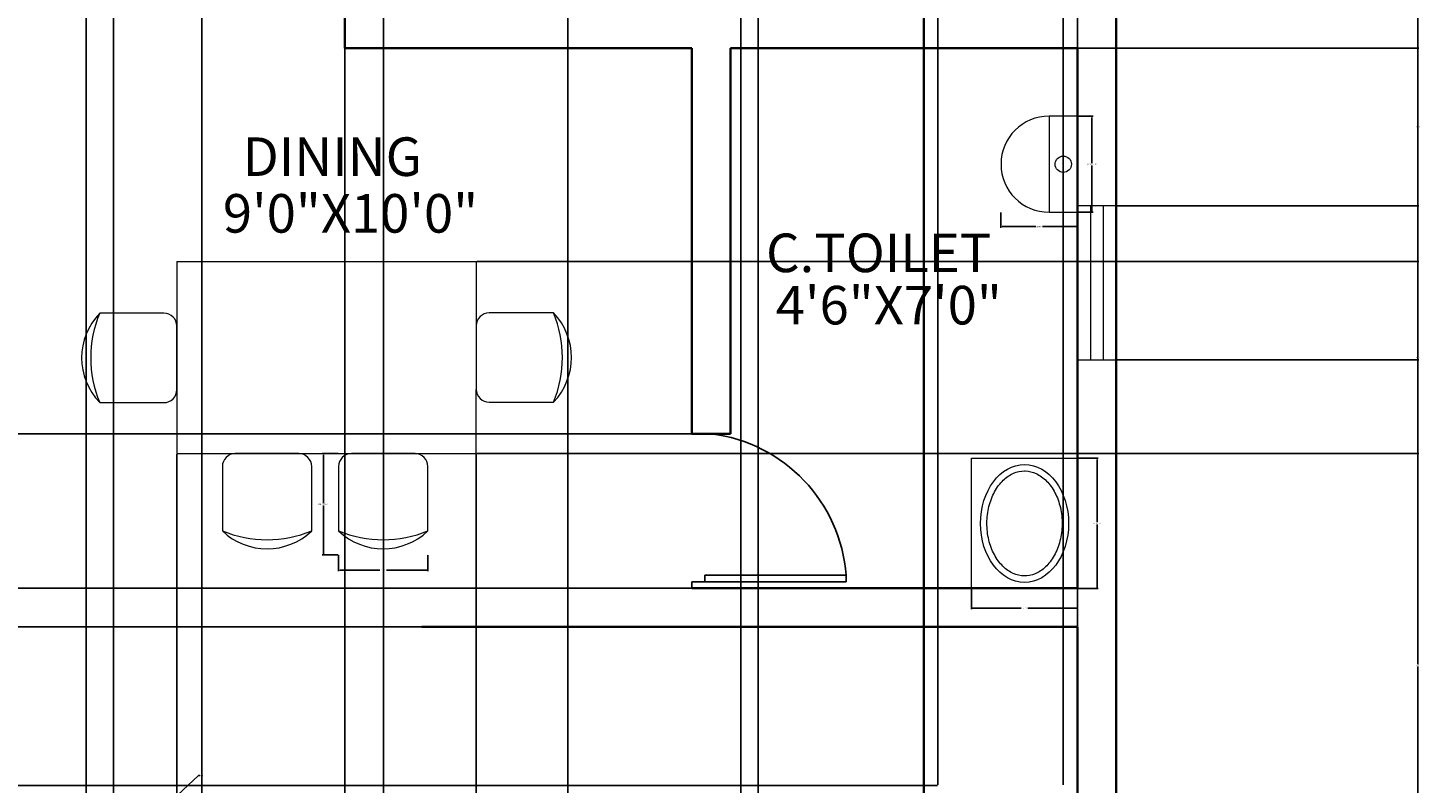
# Model space of a CAD drawing. Units: inches. Extents: x 2608 to 3003, y 1827 to 2396.
# Tile 4 of 5: x 2787 to 3003, y 2111 to 2229. Entities that reach past the tile are written whole.
import ezdxf

# ---------------------------------------------------------------- set-up
doc = ezdxf.new("R2010")
doc.units = ezdxf.units.IN
for name, color, linetype, lineweight in [('A-ANNO-DIMS', 2, 'Continuous', 18), ('A-AREA-IDEN', 7, 'Continuous', 25), ('A-DOOR', 50, 'Continuous', 25), ('A-FLOR-CASE', 213, 'Continuous', 18), ('A-FLOR-FIXT', 213, 'Continuous', 18), ('A-FURN', 254, 'Continuous', 18), ('A-GLAZ', 40, 'Continuous', 18), ('A-WALL', 111, 'Continuous', 35)]:
    doc.layers.add(name, color=color, linetype=linetype, lineweight=lineweight)
doc.styles.get("Standard").update_dxf_attribs({"font": 'arial.ttf'})
doc.dimstyles.get("Standard").update_dxf_attribs({"dimtxt": 0.18, "dimasz": 0.18, "dimexe": 0.18, "dimexo": 0.0625, "dimgap": 0.09, "dimtad": 0, "dimtih": 1, "dimtoh": 1, "dimdec": 4, "dimzin": 0, "dimdsep": 46, "dimtxsty": 'Standard', "dimcen": 0.09, "dimadec": 0, "dimazin": 0, "dimtfac": 1, "dimtdec": 4, "dimtofl": 0, "dimtmove": 0, "dimatfit": 3, "dimfxl": 1, "dimtolj": 1, "dimtzin": 0, "dimarcsym": 0})

# ---------------------------------------------------------------- blocks, each defined once
blk = doc.blocks.new('CHAIR-DINING')
blk.add_lwpolyline([(12, 13.9), (2, 13.9, 0.414214), (0, 11.9), (0, 2, 0.414214), (2, 0), (12, 0)], format="xyb")
for centre, radius, start, end in [((4.81, 6.95), 10, 315.9711, 44.0289), ((-4.6, 6.95), 18, 337.2866, 22.7134)]:
    blk.add_arc(centre, radius, start, end)
blk = doc.blocks.new('WC-PAN')
blk.add_lwpolyline([(16.51, 0), (0, 0), (0, 20.28), (16.51, 20.28)], close=True)
blk.add_ellipse((8.26, 10.14), major_axis=(0, 9.17), ratio=0.747248)
blk.add_open_spline([(8.26, 18.31), (7.68, 18.31), (7.1, 18.19), (5.98, 17.7), (5.44, 17.34), (4.44, 16.37), (3.98, 15.77), (3.23, 14.38), (2.93, 13.6), (2.52, 11.95), (2.41, 11.07), (2.4, 9.31), (2.5, 8.43), (2.9, 6.77), (3.19, 5.98), (3.94, 4.59), (4.39, 3.98), (5.38, 2.99), (5.92, 2.62), (7.04, 2.11), (7.62, 1.98), (8.77, 1.97), (9.34, 2.08), (10.47, 2.55), (11.02, 2.9), (12.02, 3.85), (12.48, 4.45), (13.25, 5.82), (13.56, 6.59), (13.98, 8.24), (14.09, 9.12), (14.12, 10.88), (14.02, 11.76), (13.64, 13.43), (13.35, 14.22), (12.62, 15.63), (12.18, 16.24), (11.19, 17.24), (10.65, 17.63), (9.53, 18.15), (8.96, 18.29), (8.34, 18.31), (8.3, 18.31), (8.26, 18.31)], degree=3, knots=[0, 0, 0, 0, 0.313014, 0.313014, 0.626027, 0.626027, 0.939041, 0.939041, 1.252055, 1.252055, 1.565069, 1.565069, 1.878082, 1.878082, 2.191096, 2.191096, 2.50411, 2.50411, 2.817124, 2.817124, 3.130137, 3.130137, 3.443151, 3.443151, 3.756165, 3.756165, 4.069179, 4.069179, 4.382192, 4.382192, 4.695206, 4.695206, 5.00822, 5.00822, 5.321234, 5.321234, 5.634247, 5.634247, 5.947261, 5.947261, 6.260275, 6.260275, 6.283185, 6.283185, 6.283185, 6.283185])
blk = doc.blocks.new('BASIN-WALL')
blk.add_lwpolyline([(11.91, 14.94), (7.47, 14.94), (7.47, 0), (11.91, 0)], close=True)
blk.add_circle((9.69, 7.47), 1.27)
blk.add_arc((7.47, 7.47), 7.47, 90, 270)
blk = doc.blocks.new('*D12')
at = {"layer": 'A-ANNO-DIMS', "color": 0, "lineweight": -2, "transparency": 16777216}
for p, q in [((2834.88, 2162.41), (2832.4, 2162.41)), ((2832.58, 2162.23), (2832.58, 2154.72)), ((2832.58, 2146.84), (2832.58, 2154.35)), ((2834.88, 2146.66), (2832.4, 2146.66))]:
    blk.add_line(p, q, dxfattribs=at)
at = {"layer": 'A-ANNO-DIMS', "color": 0, "transparency": 16777216}
for points in [[(2832.55, 2162.23), (2832.61, 2162.23), (2832.58, 2162.41)], [(2832.55, 2146.84), (2832.61, 2146.84), (2832.58, 2146.66)]]:
    blk.add_solid(points, dxfattribs=at)
at = {"layer": 'Defpoints', "color": 0, "transparency": 16777216}
for p in [(2834.94, 2162.41), (2832.58, 2146.66), (2834.94, 2146.66)]:
    blk.add_point(p, dxfattribs=at)
at = {"layer": 'A-ANNO-DIMS', "color": 0, "transparency": 16777216, "insert": (2832.58, 2154.53), "char_height": 0.18, "attachment_point": 5}
blk.add_mtext('\\A1;CHAIR 16 TYP.', dxfattribs=at)
blk = doc.blocks.new('*D13')
at = {"layer": 'A-ANNO-DIMS', "color": 0, "lineweight": -2, "transparency": 16777216}
for p, q in [((2834.94, 2146.6), (2834.94, 2144.12)), ((2848.84, 2146.6), (2848.84, 2144.12)), ((2835.12, 2144.3), (2841.37, 2144.3)), ((2848.66, 2144.3), (2842.41, 2144.3))]:
    blk.add_line(p, q, dxfattribs=at)
at = {"layer": 'A-ANNO-DIMS', "color": 0, "transparency": 16777216}
for points in [[(2835.12, 2144.33), (2835.12, 2144.27), (2834.94, 2144.3)], [(2848.66, 2144.33), (2848.66, 2144.27), (2848.84, 2144.3)]]:
    blk.add_solid(points, dxfattribs=at)
at = {"layer": 'Defpoints', "color": 0, "transparency": 16777216}
for p in [(2834.94, 2146.66), (2848.84, 2146.66), (2848.84, 2144.3)]:
    blk.add_point(p, dxfattribs=at)
at = {"layer": 'A-ANNO-DIMS', "color": 0, "transparency": 16777216, "insert": (2841.89, 2144.3), "char_height": 0.18, "attachment_point": 5}
blk.add_mtext('\\A1;14 TYP.', dxfattribs=at)
blk = doc.blocks.new('*D18')
at = {"layer": 'A-ANNO-DIMS', "color": 0, "lineweight": -2, "transparency": 16777216}
for p, q in [((2949.98, 2161.69), (2953.14, 2161.69)), ((2952.96, 2161.51), (2952.96, 2151.74)), ((2952.96, 2141.59), (2952.96, 2151.37)), ((2949.98, 2141.41), (2953.14, 2141.41))]:
    blk.add_line(p, q, dxfattribs=at)
at = {"layer": 'A-ANNO-DIMS', "color": 0, "transparency": 16777216}
for points in [[(2952.93, 2161.51), (2952.99, 2161.51), (2952.96, 2161.69)], [(2952.93, 2141.59), (2952.99, 2141.59), (2952.96, 2141.41)]]:
    blk.add_solid(points, dxfattribs=at)
at = {"layer": 'Defpoints', "color": 0, "transparency": 16777216}
for p in [(2949.92, 2161.69), (2952.96, 2161.69), (2949.92, 2141.41)]:
    blk.add_point(p, dxfattribs=at)
at = {"layer": 'A-ANNO-DIMS', "color": 0, "transparency": 16777216, "insert": (2952.96, 2151.55), "char_height": 0.18, "attachment_point": 5}
blk.add_mtext('\\A1;WC 20 TYP.', dxfattribs=at)
blk = doc.blocks.new('*D19')
at = {"layer": 'A-ANNO-DIMS', "color": 0, "lineweight": -2, "transparency": 16777216}
for p, q in [((2933.41, 2141.35), (2933.41, 2138.19)), ((2949.92, 2141.35), (2949.92, 2138.19)), ((2933.59, 2138.37), (2941.14, 2138.37)), ((2949.74, 2138.37), (2942.18, 2138.37))]:
    blk.add_line(p, q, dxfattribs=at)
at = {"layer": 'A-ANNO-DIMS', "color": 0, "transparency": 16777216}
for points in [[(2933.59, 2138.4), (2933.59, 2138.34), (2933.41, 2138.37)], [(2949.74, 2138.4), (2949.74, 2138.34), (2949.92, 2138.37)]]:
    blk.add_solid(points, dxfattribs=at)
at = {"layer": 'Defpoints', "color": 0, "transparency": 16777216}
for p in [(2933.41, 2141.41), (2949.92, 2141.41), (2949.92, 2138.37)]:
    blk.add_point(p, dxfattribs=at)
at = {"layer": 'A-ANNO-DIMS', "color": 0, "transparency": 16777216, "insert": (2941.66, 2138.37), "char_height": 0.18, "attachment_point": 5}
blk.add_mtext('\\A1;17 TYP.', dxfattribs=at)
blk = doc.blocks.new('*D20')
at = {"layer": 'A-ANNO-DIMS', "color": 0, "lineweight": -2, "transparency": 16777216}
for p, q in [((2949.98, 2214.9), (2952.34, 2214.9)), ((2952.16, 2214.72), (2952.16, 2207.61)), ((2952.16, 2200.14), (2952.16, 2207.25)), ((2949.98, 2199.96), (2952.34, 2199.96))]:
    blk.add_line(p, q, dxfattribs=at)
at = {"layer": 'A-ANNO-DIMS', "color": 0, "transparency": 16777216}
for points in [[(2952.13, 2214.72), (2952.19, 2214.72), (2952.16, 2214.9)], [(2952.13, 2200.14), (2952.19, 2200.14), (2952.16, 2199.96)]]:
    blk.add_solid(points, dxfattribs=at)
at = {"layer": 'Defpoints', "color": 0, "transparency": 16777216}
for p in [(2949.92, 2214.9), (2952.16, 2214.9), (2949.92, 2199.96)]:
    blk.add_point(p, dxfattribs=at)
at = {"layer": 'A-ANNO-DIMS', "color": 0, "transparency": 16777216, "insert": (2952.16, 2207.43), "char_height": 0.18, "attachment_point": 5}
blk.add_mtext('\\A1;BASIN 15 TYP.', dxfattribs=at)
blk = doc.blocks.new('*D21')
at = {"layer": 'A-ANNO-DIMS', "color": 0, "lineweight": -2, "transparency": 16777216}
for p, q in [((2938, 2199.9), (2938, 2197.54)), ((2949.92, 2199.9), (2949.92, 2197.54)), ((2938.18, 2197.72), (2943.44, 2197.72)), ((2949.74, 2197.72), (2944.48, 2197.72))]:
    blk.add_line(p, q, dxfattribs=at)
at = {"layer": 'A-ANNO-DIMS', "color": 0, "transparency": 16777216}
for points in [[(2938.18, 2197.75), (2938.18, 2197.69), (2938, 2197.72)], [(2949.74, 2197.75), (2949.74, 2197.69), (2949.92, 2197.72)]]:
    blk.add_solid(points, dxfattribs=at)
at = {"layer": 'Defpoints', "color": 0, "transparency": 16777216}
for p in [(2938, 2199.96), (2949.92, 2199.96), (2949.92, 2197.72)]:
    blk.add_point(p, dxfattribs=at)
at = {"layer": 'A-ANNO-DIMS', "color": 0, "transparency": 16777216, "insert": (2943.96, 2197.72), "char_height": 0.18, "attachment_point": 5}
blk.add_mtext('\\A1;12 TYP.', dxfattribs=at)
blk = doc.blocks.new('*D28')
at = {"layer": 'A-ANNO-DIMS', "color": 0, "lineweight": -2, "transparency": 16777216}
for p, q in [((2655.92, 2191.9), (2655.92, 2395.95)), ((2955.92, 2201.05), (2955.92, 2395.95)), ((2656.1, 2395.77), (2805.63, 2395.77)), ((2955.74, 2395.77), (2806.2, 2395.77))]:
    blk.add_line(p, q, dxfattribs=at)
at = {"layer": 'A-ANNO-DIMS', "color": 0, "transparency": 16777216}
for points in [[(2656.1, 2395.8), (2656.1, 2395.74), (2655.92, 2395.77)], [(2955.74, 2395.8), (2955.74, 2395.74), (2955.92, 2395.77)]]:
    blk.add_solid(points, dxfattribs=at)
at = {"layer": 'Defpoints', "color": 0, "transparency": 16777216}
for p in [(2955.92, 2395.77), (2955.92, 2200.98), (2655.92, 2191.84)]:
    blk.add_point(p, dxfattribs=at)
at = {"layer": 'A-ANNO-DIMS', "color": 0, "transparency": 16777216, "insert": (2805.92, 2395.77), "char_height": 0.18, "attachment_point": 5}
blk.add_mtext('\\A1;300', dxfattribs=at)
blk = doc.blocks.new('*D29')
at = {"layer": 'A-ANNO-DIMS', "color": 0, "lineweight": -2, "transparency": 16777216}
for p, q in [((2955.98, 2369.49), (3003.02, 2369.49)), ((3002.84, 2369.31), (3002.84, 2129.67)), ((3002.84, 1889.67), (3002.84, 2129.31)), ((2955.98, 1889.49), (3003.02, 1889.49))]:
    blk.add_line(p, q, dxfattribs=at)
at = {"layer": 'A-ANNO-DIMS', "color": 0, "transparency": 16777216}
for points in [[(3002.81, 2369.31), (3002.87, 2369.31), (3002.84, 2369.49)], [(3002.81, 1889.67), (3002.87, 1889.67), (3002.84, 1889.49)]]:
    blk.add_solid(points, dxfattribs=at)
at = {"layer": 'Defpoints', "color": 0, "transparency": 16777216}
for p in [(2955.92, 2369.49), (3002.84, 2369.49), (2955.92, 1889.49)]:
    blk.add_point(p, dxfattribs=at)
at = {"layer": 'A-ANNO-DIMS', "color": 0, "transparency": 16777216, "insert": (3002.84, 2129.49), "char_height": 0.18, "attachment_point": 5}
blk.add_mtext('\\A1;480', dxfattribs=at)
blk = doc.blocks.new('*D42')
at = {"layer": 'A-ANNO-DIMS', "color": 0, "lineweight": -2, "transparency": 16777216}
for p, q in [((2775.92, 2285.43), (2775.92, 1827.03)), ((2799.92, 2285.43), (2799.92, 1827.03)), ((2776.1, 1827.21), (2787.7, 1827.21)), ((2799.74, 1827.21), (2788.14, 1827.21))]:
    blk.add_line(p, q, dxfattribs=at)
at = {"layer": 'A-ANNO-DIMS', "color": 0, "transparency": 16777216}
for points in [[(2776.1, 1827.24), (2776.1, 1827.18), (2775.92, 1827.21)], [(2799.74, 1827.24), (2799.74, 1827.18), (2799.92, 1827.21)]]:
    blk.add_solid(points, dxfattribs=at)
at = {"layer": 'Defpoints', "color": 0, "transparency": 16777216}
for p in [(2775.92, 2285.49), (2799.92, 2285.49), (2799.92, 1827.21)]:
    blk.add_point(p, dxfattribs=at)
at = {"layer": 'A-ANNO-DIMS', "color": 0, "transparency": 16777216, "insert": (2787.92, 1827.21), "char_height": 0.18, "attachment_point": 5}
blk.add_mtext('\\A1;24', dxfattribs=at)
blk = doc.blocks.new('*D44')
at = {"layer": 'A-ANNO-DIMS', "color": 0, "lineweight": -2, "transparency": 16777216}
for p, q in [((2775.92, 2363.43), (2775.92, 1827.03)), ((2795.68, 2363.43), (2795.68, 1827.03)), ((2776.1, 1827.21), (2785.34, 1827.21)), ((2795.5, 1827.21), (2786.25, 1827.21))]:
    blk.add_line(p, q, dxfattribs=at)
at = {"layer": 'A-ANNO-DIMS', "color": 0, "transparency": 16777216}
for points in [[(2776.1, 1827.24), (2776.1, 1827.18), (2775.92, 1827.21)], [(2795.5, 1827.24), (2795.5, 1827.18), (2795.68, 1827.21)]]:
    blk.add_solid(points, dxfattribs=at)
at = {"layer": 'Defpoints', "color": 0, "transparency": 16777216}
for p in [(2775.92, 2363.49), (2795.68, 2363.49), (2795.68, 1827.21)]:
    blk.add_point(p, dxfattribs=at)
at = {"layer": 'A-ANNO-DIMS', "color": 0, "transparency": 16777216, "insert": (2785.8, 1827.21), "char_height": 0.18, "attachment_point": 5}
blk.add_mtext('\\A1;19.766', dxfattribs=at)
blk = doc.blocks.new('*D45')
at = {"layer": 'A-ANNO-DIMS', "color": 0, "lineweight": -2, "transparency": 16777216}
for p, q in [((2795.68, 2363.43), (2795.68, 1827.03)), ((2813.68, 2363.43), (2813.68, 1827.03)), ((2795.86, 1827.21), (2804.47, 1827.21)), ((2813.5, 1827.21), (2804.89, 1827.21))]:
    blk.add_line(p, q, dxfattribs=at)
at = {"layer": 'A-ANNO-DIMS', "color": 0, "transparency": 16777216}
for points in [[(2795.86, 1827.24), (2795.86, 1827.18), (2795.68, 1827.21)], [(2813.5, 1827.24), (2813.5, 1827.18), (2813.68, 1827.21)]]:
    blk.add_solid(points, dxfattribs=at)
at = {"layer": 'Defpoints', "color": 0, "transparency": 16777216}
for p in [(2795.68, 2363.49), (2813.68, 2363.49), (2813.68, 1827.21)]:
    blk.add_point(p, dxfattribs=at)
at = {"layer": 'A-ANNO-DIMS', "color": 0, "transparency": 16777216, "insert": (2804.68, 1827.21), "char_height": 0.18, "attachment_point": 5}
blk.add_mtext('\\A1;18', dxfattribs=at)
blk = doc.blocks.new('*D46')
at = {"layer": 'A-ANNO-DIMS', "color": 0, "lineweight": -2, "transparency": 16777216}
for p, q in [((2841.92, 2363.43), (2841.92, 1827.03)), ((2870.61, 2363.43), (2870.61, 1827.03)), ((2842.1, 1827.21), (2855.87, 1827.21)), ((2870.43, 1827.21), (2856.66, 1827.21))]:
    blk.add_line(p, q, dxfattribs=at)
at = {"layer": 'A-ANNO-DIMS', "color": 0, "transparency": 16777216}
for points in [[(2842.1, 1827.24), (2842.1, 1827.18), (2841.92, 1827.21)], [(2870.43, 1827.24), (2870.43, 1827.18), (2870.61, 1827.21)]]:
    blk.add_solid(points, dxfattribs=at)
at = {"layer": 'Defpoints', "color": 0, "transparency": 16777216}
for p in [(2841.92, 2363.49), (2870.61, 2363.49), (2870.61, 1827.21)]:
    blk.add_point(p, dxfattribs=at)
at = {"layer": 'A-ANNO-DIMS', "color": 0, "transparency": 16777216, "insert": (2856.26, 1827.21), "char_height": 0.18, "attachment_point": 5}
blk.add_mtext('\\A1;28.69', dxfattribs=at)
blk = doc.blocks.new('*D47')
at = {"layer": 'A-ANNO-DIMS', "color": 0, "lineweight": -2, "transparency": 16777216}
for p, q in [((2778.92, 2225.43), (2778.92, 1827.03)), ((2835.92, 2225.43), (2835.92, 1827.03)), ((2779.1, 1827.21), (2807.2, 1827.21)), ((2835.74, 1827.21), (2807.63, 1827.21))]:
    blk.add_line(p, q, dxfattribs=at)
at = {"layer": 'A-ANNO-DIMS', "color": 0, "transparency": 16777216}
for points in [[(2779.1, 1827.24), (2779.1, 1827.18), (2778.92, 1827.21)], [(2835.74, 1827.24), (2835.74, 1827.18), (2835.92, 1827.21)]]:
    blk.add_solid(points, dxfattribs=at)
at = {"layer": 'Defpoints', "color": 0, "transparency": 16777216}
for p in [(2778.92, 2225.49), (2835.92, 2225.49), (2835.92, 1827.21)]:
    blk.add_point(p, dxfattribs=at)
at = {"layer": 'A-ANNO-DIMS', "color": 0, "transparency": 16777216, "insert": (2807.42, 1827.21), "char_height": 0.18, "attachment_point": 5}
blk.add_mtext('\\A1;57', dxfattribs=at)
blk = doc.blocks.new('*D48')
at = {"layer": 'A-ANNO-DIMS', "color": 0, "lineweight": -2, "transparency": 16777216}
for p, q in [((2889.85, 2165.49), (2607.92, 2165.49)), ((2608.1, 2165.31), (2608.1, 2153.67)), ((2608.1, 2141.67), (2608.1, 2153.31)), ((2889.85, 2141.49), (2607.92, 2141.49))]:
    blk.add_line(p, q, dxfattribs=at)
at = {"layer": 'A-ANNO-DIMS', "color": 0, "transparency": 16777216}
for points in [[(2608.07, 2165.31), (2608.13, 2165.31), (2608.1, 2165.49)], [(2608.07, 2141.67), (2608.13, 2141.67), (2608.1, 2141.49)]]:
    blk.add_solid(points, dxfattribs=at)
at = {"layer": 'Defpoints', "color": 0, "transparency": 16777216}
for p in [(2608.1, 2165.49), (2889.92, 2165.49), (2889.92, 2141.49)]:
    blk.add_point(p, dxfattribs=at)
at = {"layer": 'A-ANNO-DIMS', "color": 0, "transparency": 16777216, "insert": (2608.1, 2153.49), "char_height": 0.18, "attachment_point": 5}
blk.add_mtext('\\A1;24', dxfattribs=at)
blk = doc.blocks.new('*D49')
at = {"layer": 'A-ANNO-DIMS', "color": 0, "lineweight": -2, "transparency": 16777216}
for p, q in [((2955.98, 2200.98), (3003.02, 2200.98)), ((3002.84, 2200.8), (3002.84, 2189.16)), ((3002.84, 2177.16), (3002.84, 2188.8)), ((2955.98, 2176.98), (3003.02, 2176.98))]:
    blk.add_line(p, q, dxfattribs=at)
at = {"layer": 'A-ANNO-DIMS', "color": 0, "transparency": 16777216}
for points in [[(3002.81, 2200.8), (3002.87, 2200.8), (3002.84, 2200.98)], [(3002.81, 2177.16), (3002.87, 2177.16), (3002.84, 2176.98)]]:
    blk.add_solid(points, dxfattribs=at)
at = {"layer": 'Defpoints', "color": 0, "transparency": 16777216}
for p in [(2955.92, 2200.98), (3002.84, 2200.98), (2955.92, 2176.98)]:
    blk.add_point(p, dxfattribs=at)
at = {"layer": 'A-ANNO-DIMS', "color": 0, "transparency": 16777216, "insert": (3002.84, 2188.98), "char_height": 0.18, "attachment_point": 5}
blk.add_mtext('\\A1;24', dxfattribs=at)
blk = doc.blocks.new('*D50')
at = {"layer": 'A-ANNO-DIMS', "color": 0, "lineweight": -2, "transparency": 16777216}
for p, q in [((2949.98, 2225.49), (3003.02, 2225.49)), ((3002.84, 2225.31), (3002.84, 2213.42)), ((3002.84, 2201.16), (3002.84, 2213.05)), ((2955.98, 2200.98), (3003.02, 2200.98))]:
    blk.add_line(p, q, dxfattribs=at)
at = {"layer": 'A-ANNO-DIMS', "color": 0, "transparency": 16777216}
for points in [[(3002.81, 2225.31), (3002.87, 2225.31), (3002.84, 2225.49)], [(3002.81, 2201.16), (3002.87, 2201.16), (3002.84, 2200.98)]]:
    blk.add_solid(points, dxfattribs=at)
at = {"layer": 'Defpoints', "color": 0, "transparency": 16777216}
for p in [(2949.92, 2225.49), (3002.84, 2225.49), (2955.92, 2200.98)]:
    blk.add_point(p, dxfattribs=at)
at = {"layer": 'A-ANNO-DIMS', "color": 0, "transparency": 16777216, "insert": (3002.84, 2213.24), "char_height": 0.18, "attachment_point": 5}
blk.add_mtext('\\A1;24.506', dxfattribs=at)
blk = doc.blocks.new('*D54')
at = {"layer": 'A-ANNO-DIMS', "color": 0, "lineweight": -2, "transparency": 16777216}
for p, q in [((2925.92, 2135.55), (2925.92, 2395.95)), ((2949.92, 2135.55), (2949.92, 2395.95)), ((2926.1, 2395.77), (2937.7, 2395.77)), ((2949.74, 2395.77), (2938.14, 2395.77))]:
    blk.add_line(p, q, dxfattribs=at)
at = {"layer": 'A-ANNO-DIMS', "color": 0, "transparency": 16777216}
for points in [[(2926.1, 2395.8), (2926.1, 2395.74), (2925.92, 2395.77)], [(2949.74, 2395.8), (2949.74, 2395.74), (2949.92, 2395.77)]]:
    blk.add_solid(points, dxfattribs=at)
at = {"layer": 'Defpoints', "color": 0, "transparency": 16777216}
for p in [(2949.92, 2395.77), (2925.92, 2135.49), (2949.92, 2135.49)]:
    blk.add_point(p, dxfattribs=at)
at = {"layer": 'A-ANNO-DIMS', "color": 0, "transparency": 16777216, "insert": (2937.92, 2395.77), "char_height": 0.18, "attachment_point": 5}
blk.add_mtext('\\A1;24', dxfattribs=at)
blk = doc.blocks.new('*D55')
at = {"layer": 'A-ANNO-DIMS', "color": 0, "lineweight": -2, "transparency": 16777216}
for p, q in [((2847.85, 2135.49), (2607.92, 2135.49)), ((2608.1, 2135.31), (2608.1, 2122.17)), ((2608.1, 2108.67), (2608.1, 2121.81)), ((2853.85, 2108.49), (2607.92, 2108.49))]:
    blk.add_line(p, q, dxfattribs=at)
at = {"layer": 'A-ANNO-DIMS', "color": 0, "transparency": 16777216}
for points in [[(2608.07, 2135.31), (2608.13, 2135.31), (2608.1, 2135.49)], [(2608.07, 2108.67), (2608.13, 2108.67), (2608.1, 2108.49)]]:
    blk.add_solid(points, dxfattribs=at)
at = {"layer": 'Defpoints', "color": 0, "transparency": 16777216}
for p in [(2608.1, 2135.49), (2847.92, 2135.49), (2853.92, 2108.49)]:
    blk.add_point(p, dxfattribs=at)
at = {"layer": 'A-ANNO-DIMS', "color": 0, "transparency": 16777216, "insert": (2608.1, 2121.99), "char_height": 0.18, "attachment_point": 5}
blk.add_mtext('\\A1;27', dxfattribs=at)
blk = doc.blocks.new('*D57')
at = {"layer": 'A-ANNO-DIMS', "color": 0, "lineweight": -2, "transparency": 16777216}
for p, q in [((2897.55, 2039.55), (2897.55, 2395.95)), ((2925.92, 2039.55), (2925.92, 2395.95)), ((2897.73, 2395.77), (2911.34, 2395.77)), ((2925.74, 2395.77), (2912.13, 2395.77))]:
    blk.add_line(p, q, dxfattribs=at)
at = {"layer": 'A-ANNO-DIMS', "color": 0, "transparency": 16777216}
for points in [[(2897.73, 2395.8), (2897.73, 2395.74), (2897.55, 2395.77)], [(2925.74, 2395.8), (2925.74, 2395.74), (2925.92, 2395.77)]]:
    blk.add_solid(points, dxfattribs=at)
at = {"layer": 'Defpoints', "color": 0, "transparency": 16777216}
for p in [(2925.92, 2395.77), (2897.55, 2039.49), (2925.92, 2039.49)]:
    blk.add_point(p, dxfattribs=at)
at = {"layer": 'A-ANNO-DIMS', "color": 0, "transparency": 16777216, "insert": (2911.73, 2395.77), "char_height": 0.18, "attachment_point": 5}
blk.add_mtext('\\A1;28.37', dxfattribs=at)
blk = doc.blocks.new('*D60')
at = {"layer": 'A-ANNO-DIMS', "color": 0, "lineweight": -2, "transparency": 16777216}
for p, q in [((2928.16, 2110.88), (2928.16, 2395.95)), ((2947.65, 2110.88), (2947.65, 2395.95)), ((2928.34, 2395.77), (2937.45, 2395.77)), ((2947.47, 2395.77), (2938.36, 2395.77))]:
    blk.add_line(p, q, dxfattribs=at)
at = {"layer": 'A-ANNO-DIMS', "color": 0, "transparency": 16777216}
for points in [[(2928.34, 2395.8), (2928.34, 2395.74), (2928.16, 2395.77)], [(2947.47, 2395.8), (2947.47, 2395.74), (2947.65, 2395.77)]]:
    blk.add_solid(points, dxfattribs=at)
at = {"layer": 'Defpoints', "color": 0, "transparency": 16777216}
for p in [(2947.65, 2395.77), (2928.16, 2110.81), (2947.65, 2110.81)]:
    blk.add_point(p, dxfattribs=at)
at = {"layer": 'A-ANNO-DIMS', "color": 0, "transparency": 16777216, "insert": (2937.9, 2395.77), "char_height": 0.18, "attachment_point": 5}
blk.add_mtext('\\A1;19.493', dxfattribs=at)
blk = doc.blocks.new('*D62')
at = {"layer": 'A-ANNO-DIMS', "color": 0, "lineweight": -2, "transparency": 16777216}
for p, q in [((2925.85, 2135.49), (2607.92, 2135.49)), ((2608.1, 2135.31), (2608.1, 2123.33)), ((2608.1, 2110.99), (2608.1, 2122.97)), ((2928.1, 2110.81), (2607.92, 2110.81))]:
    blk.add_line(p, q, dxfattribs=at)
at = {"layer": 'A-ANNO-DIMS', "color": 0, "transparency": 16777216}
for points in [[(2608.07, 2135.31), (2608.13, 2135.31), (2608.1, 2135.49)], [(2608.07, 2110.99), (2608.13, 2110.99), (2608.1, 2110.81)]]:
    blk.add_solid(points, dxfattribs=at)
at = {"layer": 'Defpoints', "color": 0, "transparency": 16777216}
for p in [(2925.92, 2135.49), (2608.1, 2110.81), (2928.16, 2110.81)]:
    blk.add_point(p, dxfattribs=at)
at = {"layer": 'A-ANNO-DIMS', "color": 0, "transparency": 16777216, "insert": (2608.1, 2123.15), "char_height": 0.18, "attachment_point": 5}
blk.add_mtext('\\A1;24.675', dxfattribs=at)
blk = doc.blocks.new('*D63')
at = {"layer": 'A-ANNO-DIMS', "color": 0, "lineweight": -2, "transparency": 16777216}
for p, q in [((2900.2, 2036.91), (2900.2, 2395.95)), ((2926.07, 2036.91), (2926.07, 2395.95)), ((2900.38, 2395.77), (2912.67, 2395.77)), ((2925.89, 2395.77), (2913.6, 2395.77))]:
    blk.add_line(p, q, dxfattribs=at)
at = {"layer": 'A-ANNO-DIMS', "color": 0, "transparency": 16777216}
for points in [[(2900.38, 2395.8), (2900.38, 2395.74), (2900.2, 2395.77)], [(2925.89, 2395.8), (2925.89, 2395.74), (2926.07, 2395.77)]]:
    blk.add_solid(points, dxfattribs=at)
at = {"layer": 'Defpoints', "color": 0, "transparency": 16777216}
for p in [(2926.07, 2395.77), (2900.2, 2036.85), (2926.07, 2036.85)]:
    blk.add_point(p, dxfattribs=at)
at = {"layer": 'A-ANNO-DIMS', "color": 0, "transparency": 16777216, "insert": (2913.13, 2395.77), "char_height": 0.18, "attachment_point": 5}
blk.add_mtext('\\A1;25.865', dxfattribs=at)
blk = doc.blocks.new('*D70')
at = {"layer": 'A-ANNO-DIMS', "color": 0, "lineweight": -2, "transparency": 16777216}
for p, q in [((2809.78, 2162.35), (2809.78, 1827.03)), ((2856.37, 2162.35), (2856.37, 1827.03)), ((2809.96, 1827.21), (2832.68, 1827.21)), ((2856.19, 1827.21), (2833.47, 1827.21))]:
    blk.add_line(p, q, dxfattribs=at)
at = {"layer": 'A-ANNO-DIMS', "color": 0, "transparency": 16777216}
for points in [[(2809.96, 1827.24), (2809.96, 1827.18), (2809.78, 1827.21)], [(2856.19, 1827.24), (2856.19, 1827.18), (2856.37, 1827.21)]]:
    blk.add_solid(points, dxfattribs=at)
at = {"layer": 'Defpoints', "color": 0, "transparency": 16777216}
for p in [(2809.78, 2162.41), (2856.37, 2162.41), (2856.37, 1827.21)]:
    blk.add_point(p, dxfattribs=at)
at = {"layer": 'A-ANNO-DIMS', "color": 0, "transparency": 16777216, "insert": (2833.07, 1827.21), "char_height": 0.18, "attachment_point": 5}
blk.add_mtext('\\A1;46.59', dxfattribs=at)
blk = doc.blocks.new('*D71')
at = {"layer": 'A-ANNO-DIMS', "color": 0, "lineweight": -2, "transparency": 16777216}
for p, q in [((2856.43, 2192.31), (3003.02, 2192.31)), ((3002.84, 2192.13), (3002.84, 2177.54)), ((3002.84, 2162.59), (3002.84, 2177.18)), ((2856.43, 2162.41), (3003.02, 2162.41))]:
    blk.add_line(p, q, dxfattribs=at)
at = {"layer": 'A-ANNO-DIMS', "color": 0, "transparency": 16777216}
for points in [[(3002.81, 2192.13), (3002.87, 2192.13), (3002.84, 2192.31)], [(3002.81, 2162.59), (3002.87, 2162.59), (3002.84, 2162.41)]]:
    blk.add_solid(points, dxfattribs=at)
at = {"layer": 'Defpoints', "color": 0, "transparency": 16777216}
for p in [(2856.37, 2192.31), (3002.84, 2192.31), (2856.37, 2162.41)]:
    blk.add_point(p, dxfattribs=at)
at = {"layer": 'A-ANNO-DIMS', "color": 0, "transparency": 16777216, "insert": (3002.84, 2177.36), "char_height": 0.18, "attachment_point": 5}
blk.add_mtext('\\A1;29.9', dxfattribs=at)
blk = doc.blocks.new('*D76')
at = {"layer": 'A-ANNO-DIMS', "color": 0, "lineweight": -2, "transparency": 16777216}
for p, q in [((2813.16, 2112.32), (2794.82, 2095.3)), ((2813.34, 2112.32), (2813.16, 2112.32)), ((2763.83, 2066.6), (2764.01, 2066.6)), ((2763.92, 2066.51), (2763.92, 2066.69))]:
    blk.add_line(p, q, dxfattribs=at)
at = {"layer": 'A-ANNO-DIMS', "color": 0, "transparency": 16777216}
blk.add_solid([(2794.8, 2095.32), (2794.85, 2095.28), (2794.69, 2095.18)], dxfattribs=at)
at = {"layer": 'Defpoints', "color": 0, "transparency": 16777216}
for p in [(2794.69, 2095.18), (2763.92, 2066.6)]:
    blk.add_point(p, dxfattribs=at)
at = {"layer": 'A-ANNO-DIMS', "color": 0, "transparency": 16777216, "insert": (2813.64, 2112.32), "char_height": 0.18, "attachment_point": 5}
blk.add_mtext('\\A1;R42', dxfattribs=at)

msp = doc.modelspace()

# ---------------------------------------------------------------- linework, layer by layer
at = {"layer": 'A-DOOR'}
for p, q in [((2889.9155, 2141.4896), (2889.9155, 2142.4896)), ((2889.9155, 2142.4896), (2913.9155, 2142.4896)), ((2913.9155, 2143.4896), (2891.9155, 2143.4896)), ((2891.9155, 2143.4896), (2891.9155, 2142.4896)), ((2913.9155, 2142.4896), (2913.9155, 2143.4896))]:
    msp.add_line(p, q, dxfattribs=at)
msp.add_arc((2889.9847, 2141.6692), 24, 4.349991, 82.985569, dxfattribs=at)
at = {"layer": 'A-FLOR-CASE'}
msp.add_line((2925.9155, 2135.4896), (2925.9155, 2039.4896), dxfattribs=at)
at = {"layer": 'A-FURN'}
for p, q in [((2809.7764, 2192.3086), (2856.3703, 2192.3086)), ((2809.7764, 2192.3086), (2809.7764, 2162.4082)), ((2856.3703, 2192.3086), (2856.3703, 2182.3086)), ((2856.3703, 2162.4082), (2856.3703, 2172.4082)), ((2809.7764, 2162.4082), (2856.3703, 2162.4082))]:
    msp.add_line(p, q, dxfattribs=at)
at = {"layer": 'A-GLAZ'}
for p, q in [((2949.9155, 2200.9836), (2955.9155, 2200.9836)), ((2951.9155, 2200.9836), (2951.9155, 2176.9836)), ((2953.9155, 2200.9836), (2953.9155, 2176.9836)), ((2949.9155, 2176.9836), (2955.9155, 2176.9836))]:
    msp.add_line(p, q, dxfattribs=at)
at = {"layer": 'A-WALL'}
for p, q in [((2835.9155, 2225.4896), (2835.9155, 2237.4896)), ((2835.9155, 2225.4896), (2889.9155, 2225.4896)), ((2889.9155, 2225.4896), (2889.9155, 2165.4896)), ((2895.9155, 2225.4896), (2895.9155, 2165.4896)), ((2895.9155, 2225.4896), (2949.9155, 2225.4896)), ((2949.9155, 2225.4896), (2949.9155, 2141.4896)), ((2889.9155, 2165.4896), (2895.9155, 2165.4896)), ((2889.9155, 2141.4896), (2949.9155, 2141.4896)), ((2847.9155, 2135.4896), (2949.9155, 2135.4896)), ((2949.9155, 2135.4896), (2949.9155, 2015.4896))]:
    msp.add_line(p, q, dxfattribs=at)
msp.add_lwpolyline([(2655.9155, 2369.4896), (2955.9155, 2369.4896), (2955.9155, 1889.4896), (2655.9155, 1889.4896)], close=True, dxfattribs=at)

# ---------------------------------------------------------------- block references
at = {"layer": 'A-FLOR-FIXT'}
for name, p in [('BASIN-WALL', (2938.005, 2199.9632)), ('WC-PAN', (2933.405, 2141.4105))]:
    msp.add_blockref(name, p, dxfattribs=at)
at = {"layer": 'A-FURN'}
for p, rotation in [((2809.7767, 2184.2477), 180), ((2816.8581, 2162.4085), 269.9999999999992), ((2834.9374, 2162.4085), 269.9999999999974)]:
    msp.add_blockref('CHAIR-DINING', p, dxfattribs=dict(at, rotation=rotation))
msp.add_blockref('CHAIR-DINING', (2856.37, 2170.408), dxfattribs=at)

# ---------------------------------------------------------------- texts
at = {"layer": 'A-AREA-IDEN'}
for tag, p in [('DINING', (2820.0066, 2205.6041)), ('9\'0"X10\'0"', (2816.9383, 2196.7862)), ('C.TOILET', (2901.4482, 2190.6397)), ('4\'6"X7\'0"', (2902.9596, 2182.5084))]:
    msp.add_attdef(tag, p, '', height=6, dxfattribs=at)

# ---------------------------------------------------------------- dimensions: what is measured, and where the dimension line sits
at = {"layer": 'A-ANNO-DIMS'}
for base, p1, p2, override, picture, middle in [((2955.9155, 2395.7696), (2655.9155, 2191.8395), (2955.9155, 2200.9836), {"dimdec": 0, "dimlfac": 1, "dimrnd": 0, "dimzin": 0, "dimdsep": 46, "dimlunit": 2}, '*D28', (2805.9155, 2395.7696)), ((2925.9155, 2395.7696), (2897.5458, 2039.4896), (2925.9155, 2039.4896), {"dimdec": 2, "dimlfac": 1, "dimrnd": 0, "dimzin": 0, "dimdsep": 46, "dimlunit": 2}, '*D57', (2911.7307, 2395.7696)), ((2926.0657, 2395.7696), (2900.2006, 2036.8464), (2926.0657, 2036.8464), {"dimdec": 3, "dimlfac": 1, "dimrnd": 0, "dimzin": 0, "dimdsep": 46, "dimlunit": 2}, '*D63', (2913.1332, 2395.7696)), ((2949.9155, 2395.7696), (2925.9155, 2135.4896), (2949.9155, 2135.4896), {"dimdec": 0, "dimlfac": 1, "dimrnd": 0, "dimzin": 0, "dimdsep": 46, "dimlunit": 2}, '*D54', (2937.9155, 2395.7696)), ((2947.6506, 2395.7696), (2928.1576, 2110.8146), (2947.6506, 2110.8146), {"dimdec": 3, "dimlfac": 1, "dimrnd": 0, "dimzin": 0, "dimdsep": 46, "dimlunit": 2}, '*D60', (2937.9041, 2395.7696)), ((2795.6817, 1827.2096), (2775.9155, 2363.4896), (2795.6817, 2363.4896), {"dimdec": 3, "dimlfac": 1, "dimrnd": 0, "dimzin": 0, "dimdsep": 46, "dimlunit": 2}, '*D44', (2785.7986, 1827.2096)), ((2813.6817, 1827.2096), (2795.6817, 2363.4896), (2813.6817, 2363.4896), {"dimdec": 0, "dimlfac": 1, "dimrnd": 0, "dimzin": 0, "dimdsep": 46, "dimlunit": 2}, '*D45', (2804.6817, 1827.2096)), ((2870.6078, 1827.2096), (2841.9155, 2363.4896), (2870.6078, 2363.4896), {"dimdec": 2, "dimlfac": 1, "dimrnd": 0, "dimzin": 0, "dimdsep": 46, "dimlunit": 2}, '*D46', (2856.2616, 1827.2096)), ((2799.9155, 1827.2096), (2775.9155, 2285.4896), (2799.9155, 2285.4896), {"dimdec": 0, "dimlfac": 1, "dimrnd": 0, "dimzin": 0, "dimdsep": 46, "dimlunit": 2}, '*D42', (2787.9155, 1827.2096)), ((2835.9155, 1827.2096), (2778.9155, 2225.4896), (2835.9155, 2225.4896), {"dimdec": 0, "dimlfac": 1, "dimrnd": 0, "dimzin": 0, "dimdsep": 46, "dimlunit": 2}, '*D47', (2807.4155, 1827.2096)), ((2856.3703, 1827.2096), (2809.7764, 2162.4082), (2856.3703, 2162.4082), {"dimdec": 2, "dimlfac": 1, "dimrnd": 0, "dimzin": 0, "dimdsep": 46, "dimlunit": 2}, '*D70', (2833.0733, 1827.2096))]:
    dim = msp.add_linear_dim(base=base, p1=p1, p2=p2, dimstyle='Standard', override=override, dxfattribs=at)
    dim.commit()
    dim.dimension.update_dxf_attribs({"geometry": picture, "text_midpoint": middle})
for base, p1, p2, override, picture, middle in [((3002.8414, 2369.4896), (2955.9155, 1889.4896), (2955.9155, 2369.4896), {"dimdec": 0, "dimlfac": 1, "dimrnd": 0, "dimzin": 0, "dimdsep": 46, "dimlunit": 2}, '*D29', (3002.8414, 2129.4896)), ((3002.8414, 2225.4896), (2955.9155, 2200.9836), (2949.9155, 2225.4896), {"dimdec": 3, "dimlfac": 1, "dimrnd": 0, "dimzin": 0, "dimdsep": 46, "dimlunit": 2}, '*D50', (3002.8414, 2213.2366)), ((3002.8414, 2200.9836), (2955.9155, 2176.9836), (2955.9155, 2200.9836), {"dimdec": 0, "dimlfac": 1, "dimrnd": 0, "dimzin": 0, "dimdsep": 46, "dimlunit": 2}, '*D49', (3002.8414, 2188.9836)), ((3002.8414, 2192.3086), (2856.3703, 2162.4082), (2856.3703, 2192.3086), {"dimdec": 1, "dimlfac": 1, "dimrnd": 0, "dimzin": 0, "dimdsep": 46, "dimlunit": 2}, '*D71', (3002.8414, 2177.3584)), ((2608.0955, 2165.4896), (2889.9155, 2141.4896), (2889.9155, 2165.4896), {"dimdec": 0, "dimlfac": 1, "dimrnd": 0, "dimzin": 0, "dimdsep": 46, "dimlunit": 2}, '*D48', (2608.0955, 2153.4896)), ((2608.0955, 2110.8146), (2925.9155, 2135.4896), (2928.1576, 2110.8146), {"dimdec": 3, "dimlfac": 1, "dimrnd": 0, "dimzin": 0, "dimdsep": 46, "dimlunit": 2}, '*D62', (2608.0955, 2123.1521)), ((2608.0955, 2135.4896), (2853.9155, 2108.4896), (2847.9155, 2135.4896), {"dimdec": 0, "dimlfac": 1, "dimrnd": 0, "dimzin": 0, "dimdsep": 46, "dimlunit": 2}, '*D55', (2608.0955, 2121.9896))]:
    dim = msp.add_linear_dim(base=base, p1=p1, p2=p2, angle=90, dimstyle='Standard', override=override, dxfattribs=at)
    dim.commit()
    dim.dimension.update_dxf_attribs({"geometry": picture, "text_midpoint": middle})
for base, p1, p2, angle, text, picture, middle in [((2952.1561, 2214.9004), (2949.9155, 2199.9631), (2949.9155, 2214.9004), 90, 'BASIN <> TYP.', '*D20', (2952.1561, 2207.4318)), ((2832.5756, 2146.6614), (2834.9376, 2162.4082), (2834.9376, 2146.6614), 270, 'CHAIR <> TYP.', '*D12', (2832.5756, 2154.5348)), ((2952.9582, 2161.6945), (2949.9155, 2141.4101), (2949.9155, 2161.6945), 90, 'WC <> TYP.', '*D18', (2952.9582, 2151.5523))]:
    dim = msp.add_linear_dim(base=base, p1=p1, p2=p2, angle=angle, text=text, dimstyle='Standard', override={"dimdec": 0, "dimlfac": 1, "dimrnd": 0, "dimzin": 0, "dimdsep": 46, "dimlunit": 2}, dxfattribs=at)
    dim.commit()
    dim.dimension.update_dxf_attribs({"geometry": picture, "text_midpoint": middle})
for base, p1, p2, picture, middle in [((2949.9155, 2197.7226), (2938.0049, 2199.9631), (2949.9155, 2199.9631), '*D21', (2943.9602, 2197.7226)), ((2848.838, 2144.2994), (2834.9376, 2146.6614), (2848.838, 2146.6614), '*D13', (2841.8878, 2144.2994)), ((2949.9155, 2138.3675), (2933.4054, 2141.4101), (2949.9155, 2141.4101), '*D19', (2941.6605, 2138.3675))]:
    dim = msp.add_linear_dim(base=base, p1=p1, p2=p2, text='<> TYP.', dimstyle='Standard', override={"dimdec": 0, "dimlfac": 1, "dimrnd": 0, "dimzin": 0, "dimdsep": 46, "dimlunit": 2}, dxfattribs=at)
    dim.commit()
    dim.dimension.update_dxf_attribs({"geometry": picture, "text_midpoint": middle})
dim = msp.add_radius_dim(center=(2763.9157, 2066.5969), mpoint=(2794.6929, 2095.1759), dimstyle='Standard', override={"dimdec": 0, "dimlfac": 1, "dimrnd": 0, "dimzin": 0, "dimdsep": 46, "dimlunit": 2}, dxfattribs=at)
dim.commit()
dim.dimension.update_dxf_attribs({"geometry": '*D76', "text_midpoint": (2813.6434, 2112.3233), "dimtype": 164})

doc.saveas('drawing.dxf')
